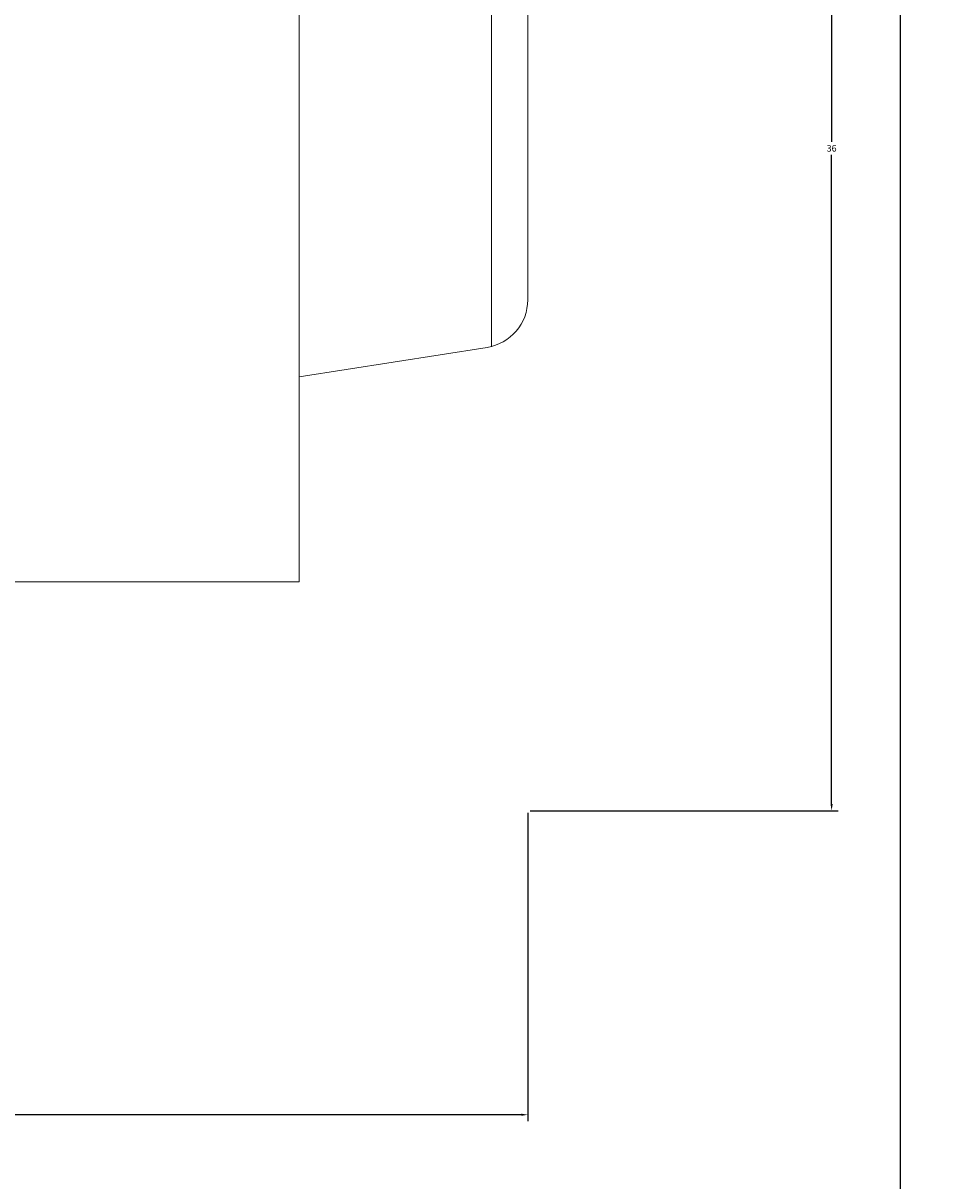
# Model space of a CAD drawing. Units: inches. Extents: x 2231 to 2461, y 2045 to 2455.
# Tile 25 of 95: x 2371 to 2396, y 2112 to 2144. Entities that reach past the tile are written whole.
import ezdxf

# ---------------------------------------------------------------- set-up
doc = ezdxf.new("R2010")
doc.units = ezdxf.units.IN
doc.layers.add('A-ANNO-DIMS', color=2, linetype='Continuous', lineweight=18)
doc.layers.add('A-FURN', color=9, linetype='Continuous', lineweight=18)
doc.styles.get("Standard").update_dxf_attribs({"font": 'arial.ttf'})
doc.dimstyles.get("Standard").update_dxf_attribs({"dimtxt": 0.18, "dimasz": 0.18, "dimexe": 0.18, "dimexo": 0.0625, "dimgap": 0.09, "dimtad": 0, "dimtih": 1, "dimtoh": 1, "dimdec": 4, "dimzin": 0, "dimdsep": 46, "dimtxsty": 'Standard', "dimcen": 0.09, "dimadec": 0, "dimazin": 0, "dimtfac": 1, "dimtdec": 4, "dimtofl": 0, "dimtmove": 0, "dimatfit": 3, "dimfxl": 1, "dimtolj": 1, "dimtzin": 0, "dimarcsym": 0})

# ---------------------------------------------------------------- blocks, each defined once
blk = doc.blocks.new('Dining Set - 36 x 72 in.')
for p, q in [((29.162, -18), (29.162, 18)), ((37.162, 8.23), (37.162, -8.239)), ((38.662, 6.288), (38.662, -6.288)), ((29.16, -9.485), (36.971, -8.264)), ((-4.062, -18), (29.162, -18))]:
    blk.add_line(p, q)
blk.add_arc((36.662, -6.288), 2, 278.8806, 0)
blk = doc.blocks.new('*D31')
at = {"layer": 'A-ANNO-DIMS', "color": 0, "lineweight": -2, "transparency": 16777216}
for p, q in [((2328.765, 2122.602), (2328.765, 2114.118)), ((2384.543, 2122.602), (2384.543, 2114.118)), ((2328.945, 2114.298), (2355.685, 2114.298)), ((2384.363, 2114.298), (2357.623, 2114.298))]:
    blk.add_line(p, q, dxfattribs=at)
at = {"layer": 'A-ANNO-DIMS', "color": 0, "transparency": 16777216}
for points in [[(2328.945, 2114.328), (2328.945, 2114.268), (2328.765, 2114.298)], [(2384.363, 2114.328), (2384.363, 2114.268), (2384.543, 2114.298)]]:
    blk.add_solid(points, dxfattribs=at)
at = {"layer": 'Defpoints', "color": 0, "transparency": 16777216}
for p in [(2328.765, 2122.665), (2384.543, 2122.665), (2384.543, 2114.298)]:
    blk.add_point(p, dxfattribs=at)
at = {"layer": 'A-ANNO-DIMS', "color": 0, "transparency": 16777216, "insert": (2356.654, 2114.298), "char_height": 0.18, "attachment_point": 5}
blk.add_mtext('\\A1;DINING SET 56', dxfattribs=at)
blk = doc.blocks.new('*D32')
at = {"layer": 'A-ANNO-DIMS', "color": 0, "lineweight": -2, "transparency": 16777216}
for p, q in [((2384.605, 2159.115), (2393.089, 2159.115)), ((2392.909, 2158.935), (2392.909, 2141.072)), ((2392.909, 2122.845), (2392.909, 2140.708)), ((2384.605, 2122.665), (2393.089, 2122.665))]:
    blk.add_line(p, q, dxfattribs=at)
at = {"layer": 'A-ANNO-DIMS', "color": 0, "transparency": 16777216}
for points in [[(2392.879, 2158.935), (2392.939, 2158.935), (2392.909, 2159.115)], [(2392.879, 2122.845), (2392.939, 2122.845), (2392.909, 2122.665)]]:
    blk.add_solid(points, dxfattribs=at)
at = {"layer": 'Defpoints', "color": 0, "transparency": 16777216}
for p in [(2384.543, 2159.115), (2392.909, 2159.115), (2384.543, 2122.665)]:
    blk.add_point(p, dxfattribs=at)
at = {"layer": 'A-ANNO-DIMS', "color": 0, "transparency": 16777216, "insert": (2392.909, 2140.89), "char_height": 0.18, "attachment_point": 5}
blk.add_mtext('\\A1;36', dxfattribs=at)
blk = doc.blocks.new('*D66')
at = {"layer": 'A-ANNO-DIMS', "color": 0, "lineweight": -2, "transparency": 16777216}
for p, q in [((2348.189, 2096.895), (2348.189, 2454.645)), ((2348.369, 2454.465), (2378.167, 2454.465)), ((2408.614, 2454.465), (2378.815, 2454.465)), ((2408.794, 2096.895), (2408.794, 2454.645))]:
    blk.add_line(p, q, dxfattribs=at)
at = {"layer": 'A-ANNO-DIMS', "color": 0, "transparency": 16777216}
for points in [[(2348.369, 2454.495), (2348.369, 2454.435), (2348.189, 2454.465)], [(2408.614, 2454.495), (2408.614, 2454.435), (2408.794, 2454.465)]]:
    blk.add_solid(points, dxfattribs=at)
at = {"layer": 'Defpoints', "color": 0, "transparency": 16777216}
for p in [(2408.794, 2454.465), (2348.189, 2096.833), (2408.794, 2096.833)]:
    blk.add_point(p, dxfattribs=at)
at = {"layer": 'A-ANNO-DIMS', "color": 0, "transparency": 16777216, "insert": (2378.491, 2454.465), "char_height": 0.18, "attachment_point": 5}
blk.add_mtext('\\A1;60.6', dxfattribs=at)
blk = doc.blocks.new('*D69')
at = {"layer": 'A-ANNO-DIMS', "color": 0, "lineweight": -2, "transparency": 16777216}
for p, q in [((2340.667, 2189.285), (2340.667, 2044.803)), ((2394.794, 2186.77), (2394.794, 2044.803)), ((2340.847, 2044.983), (2367.337, 2044.983)), ((2394.614, 2044.983), (2368.124, 2044.983))]:
    blk.add_line(p, q, dxfattribs=at)
at = {"layer": 'A-ANNO-DIMS', "color": 0, "transparency": 16777216}
for points in [[(2340.847, 2045.013), (2340.847, 2044.953), (2340.667, 2044.983)], [(2394.614, 2045.013), (2394.614, 2044.953), (2394.794, 2044.983)]]:
    blk.add_solid(points, dxfattribs=at)
at = {"layer": 'Defpoints', "color": 0, "transparency": 16777216}
for p in [(2340.667, 2189.348), (2394.794, 2186.833), (2394.794, 2044.983)]:
    blk.add_point(p, dxfattribs=at)
at = {"layer": 'A-ANNO-DIMS', "color": 0, "transparency": 16777216, "insert": (2367.73, 2044.983), "char_height": 0.18, "attachment_point": 5}
blk.add_mtext('\\A1;54.13', dxfattribs=at)

msp = doc.modelspace()

# ---------------------------------------------------------------- block references
at = {"layer": 'A-FURN', "xscale": 0.6627357546055535, "yscale": 0.6627357546055535, "zscale": 0.6627357546055535}
msp.add_blockref('Dining Set - 36 x 72 in.', (2358.9199, 2140.8902), dxfattribs=at)

# ---------------------------------------------------------------- dimensions: what is measured, and where the dimension line sits
at = {"layer": 'A-ANNO-DIMS'}
for base, p1, p2, override, picture, middle in [((2408.7935, 2454.4653), (2348.1888, 2096.8328), (2408.7935, 2096.8328), {"dimdec": 1, "dimlfac": 1, "dimrnd": 0, "dimzin": 0, "dimdsep": 46, "dimlunit": 2}, '*D66', (2378.4912, 2454.4653)), ((2394.7935, 2044.9825), (2340.6673, 2189.3477), (2394.7935, 2186.8328), {"dimdec": 2, "dimlfac": 1, "dimrnd": 0, "dimzin": 0, "dimdsep": 46, "dimlunit": 2}, '*D69', (2367.7304, 2044.9825))]:
    dim = msp.add_linear_dim(base=base, p1=p1, p2=p2, dimstyle='Standard', override=override, dxfattribs=at)
    dim.commit()
    dim.dimension.update_dxf_attribs({"geometry": picture, "text_midpoint": middle})
dim = msp.add_linear_dim(base=(2392.9094, 2159.1154), p1=(2384.5428, 2122.665), p2=(2384.5428, 2159.1154), angle=90, dimstyle='Standard', override={"dimdec": 0, "dimlfac": 1, "dimrnd": 0, "dimzin": 0, "dimdsep": 46, "dimlunit": 2}, dxfattribs=at)
dim.commit()
dim.dimension.update_dxf_attribs({"geometry": '*D32', "text_midpoint": (2392.9094, 2140.8902)})
dim = msp.add_linear_dim(base=(2384.5428, 2114.2984), p1=(2328.7655, 2122.665), p2=(2384.5428, 2122.665), text='DINING SET <>', dimstyle='Standard', override={"dimdec": 0, "dimlfac": 1, "dimrnd": 0, "dimzin": 0, "dimdsep": 46, "dimlunit": 2}, dxfattribs=at)
dim.commit()
dim.dimension.update_dxf_attribs({"geometry": '*D31', "text_midpoint": (2356.6542, 2114.2984)})

doc.saveas('drawing.dxf')
